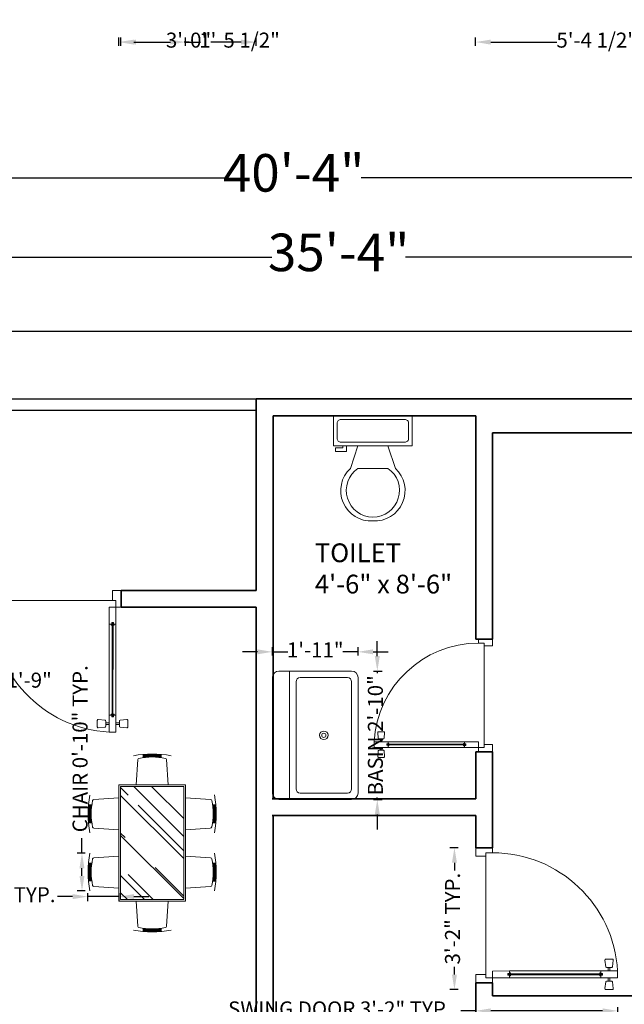
# Model space of a CAD drawing. Units: inches. Extents: x -638 to 186, y -762 to 59.
# Tile 21 of 31: x -287 to -125, y -203 to 59. Entities that reach past the tile are written whole.
import ezdxf

# ---------------------------------------------------------------- set-up
doc = ezdxf.new("R2010")
doc.units = ezdxf.units.IN
for name, color, linetype, lineweight in [('A-ANNO-DIMS', 2, 'Continuous', 18), ('A-AREA-IDEN', 1, 'Continuous', 18), ('A-DOOR', 3, 'Continuous', 18), ('A-FLOR-EDGE', 1, 'Continuous', 25), ('A-FLOR-FIXT', 9, 'Continuous', 18), ('A-FURN-PATT', 8, 'Continuous', 9), ('C-PROP', 7, 'Continuous', 25), ('furn', 8, 'Continuous', 13), ('wall', 7, 'Continuous', 35)]:
    doc.layers.add(name, color=color, linetype=linetype, lineweight=lineweight)
doc.styles.get("Standard").update_dxf_attribs({"font": 'arial.ttf'})
doc.dimstyles.new('ISO-25', dxfattribs={"dimtxt": 4, "dimasz": 4, "dimexe": 1.25, "dimexo": 0.625, "dimtad": 0, "dimlunit": 4, "dimtxsty": 'Standard', "dimcen": 2.5, "dimclrt": 256, "dimadec": 0, "dimazin": 0, "dimtfac": 1, "dimtmove": 0, "dimatfit": 3, "dimfxl": 1, "dimfxlon": 1, "dimarcsym": 0})

# ---------------------------------------------------------------- blocks, each defined once
blk = doc.blocks.new('*U4')
for p, q in [((9.5, -6), (9.5, -2)), ((-10, -8.5), (-8, -8.5)), ((-10, -9.5), (-10, -8.5)), ((-7, -9.5), (-10, -9.5)), ((-8, -8.5), (-8, -8)), ((-7, -8), (-7, -9.5)), ((-4, -8), (-6, -14)), ((4, -8), (6, -14)), ((4, -14), (-4, -14))]:
    blk.add_line(p, q)
blk.add_lwpolyline([(10.5, -8), (10.5, 0), (-10.5, 0), (-10.5, -8)], close=True)
for points in [[(-9.5, -2), (-9.5, -6)], [(8.5, -1), (-8.5, -1)], [(-8.5, -7), (8.5, -7)]]:
    blk.add_lwpolyline(points)
for centre, radius, start, end in [((-8.625, -1.875), 0.8839, 81.8699, 188.1301), ((8.625, -1.875), 0.8839, 351.8699, 98.1301), ((-8.625, -6.125), 0.8839, 171.869898, 278.1301), ((8.625, -6.125), 0.8839, 261.8699, 8.1301), ((-0.4772, -19.9188), 8.0953, 133.01722, 273.38), ((0.0374, -19.8731), 7.127, 124.50543, 269.7), ((-0.0373, -19.8731), 7.127, 270.3, 55.4946), ((0.4773, -19.9188), 8.0953, 266.62, 46.9828)]:
    blk.add_arc(centre, radius, start, end)
blk = doc.blocks.new('Sink-single - 30 in top')
blk.add_line((-15, -3.999996), (15, -3.999996))
for points in [[(-13.5, 0), (13.5, 0)], [(-15, -18.499996), (-15, -1.5)], [(15, -1.5), (15, -18.499996)], [(-13.5, -17.499996), (-13.5, -6.499996)], [(-12.5, -5.499996), (12.5, -5.499996)], [(13.5, -6.499996), (13.5, -17.499996)], [(13.5, -19.999996), (-13.5, -19.999996)], [(12.5, -18.499996), (-12.5, -18.499996)]]:
    blk.add_lwpolyline(points)
for radius in [1, 0.5]:
    blk.add_circle((0, -11.999996), radius)
for centre, radius, start, end in [((-13.5, -1.5), 1.5, 90, 180), ((13.5, -1.5), 1.5, 0, 90), ((-12.5, -6.499996), 1, 90, 180), ((12.5, -6.499996), 1, 0, 90), ((-12.5, -17.499996), 1, 180, 270), ((12.5, -17.499996), 1, 270, 0), ((-13.5, -18.499996), 1.5, 180, 270), ((13.5, -18.499996), 1.5, 270, 0)]:
    blk.add_arc(centre, radius, start, end)
blk = doc.blocks.new('*D9')
at = {"layer": 'A-ANNO-DIMS', "color": 0, "lineweight": -2, "transparency": 16777216}
for p, q in [((-413.53, -5.3), (-413.53, -3.05)), ((-403.53, -4.3), (-219.32, -4.3)), ((0.47, -4.3), (-183.73, -4.3)), ((10.47, -5.3), (10.47, -3.05))]:
    blk.add_line(p, q, dxfattribs=at)
at = {"layer": 'A-ANNO-DIMS', "color": 0, "lineweight": 30, "transparency": 16777216}
for points in [[(-403.53, -2.64), (-403.53, -5.97), (-413.53, -4.3)], [(0.47, -2.64), (0.47, -5.97), (10.47, -4.3)]]:
    blk.add_solid(points, dxfattribs=at)
at = {"layer": 'Defpoints', "color": 0, "lineweight": 30, "transparency": 16777216}
for p in [(10.47, -4.3), (-413.53, -42.03), (10.47, -42.03)]:
    blk.add_point(p, dxfattribs=at)
at = {"layer": 'A-ANNO-DIMS', "color": 0, "transparency": 16777216, "insert": (-201.53, -4.3), "char_height": 10, "attachment_point": 5}
blk.add_mtext('35\'-4"', dxfattribs=at)
blk = doc.blocks.new('*D11')
at = {"layer": 'A-ANNO-DIMS', "color": 0, "lineweight": -2, "transparency": 16777216}
for p, q in [((-455.53, 15.89), (-455.53, 18.14)), ((-445.53, 16.89), (-231.53, 16.89)), ((18.47, 16.89), (-195.52, 16.89)), ((28.47, 15.89), (28.47, 18.14))]:
    blk.add_line(p, q, dxfattribs=at)
at = {"layer": 'A-ANNO-DIMS', "color": 0, "lineweight": 30, "transparency": 16777216}
for points in [[(-445.53, 18.56), (-445.53, 15.23), (-455.53, 16.89)], [(18.47, 18.56), (18.47, 15.23), (28.47, 16.89)]]:
    blk.add_solid(points, dxfattribs=at)
at = {"layer": 'Defpoints', "color": 0, "lineweight": 30, "transparency": 16777216}
for p in [(28.47, 16.89), (-455.53, -42.03), (28.47, -42.03)]:
    blk.add_point(p, dxfattribs=at)
at = {"layer": 'A-ANNO-DIMS', "color": 0, "transparency": 16777216, "insert": (-213.53, 16.89), "char_height": 10, "attachment_point": 5}
blk.add_mtext('40\'-4"', dxfattribs=at)
blk = doc.blocks.new('DOOR-SWING-36IN')
for p, q in [((35.54, 35.1), (4.05, 35.09)), ((3.95, 4.05), (3.94, 29.24)), ((4.06, 4.05), (4.06, 29.24)), ((4.18, 4.05), (4.17, 29.24)), ((3.16, 4.5), (3.16, 28.79)), ((4.96, 4.5), (4.96, 28.79))]:
    blk.add_line(p, q)
for points in [[(3.16, 33.29), (3.15, 35.09), (4.05, 35.09), (4.05, 37.78), (1.8, 37.78), (1.81, 33.29), (3.16, 33.29)], [(36.44, 33.3), (36.44, 35.1), (35.54, 35.1), (35.54, 37.79), (37.79, 37.8), (37.79, 33.3), (36.44, 33.3)], [(4.28, 28.79), (4.96, 28.79), (4.95, 33.29), (3.16, 33.29), (3.16, 28.79), (3.83, 28.79), (3.83, 29.24), (4.28, 29.24), (4.28, 28.79)], [(4.29, 4.5), (4.96, 4.5), (4.96, 0), (3.17, 0), (3.16, 4.5), (3.84, 4.5), (3.84, 4.05), (4.29, 4.05), (4.29, 4.5)]]:
    blk.add_lwpolyline(points)
for points in [[(2.05, 3.17), (0.25, 3.35, 0.443716), (0, 3.12), (0, 1.37, 0.443716), (0.25, 1.15), (2.05, 1.33, 0.385314), (2.25, 1.55), (2.25, 2.94, 0.385314)], [(6.08, 3.17), (7.88, 3.35, -0.443716), (8.13, 3.13), (8.13, 1.37, -0.443716), (7.88, 1.15), (6.08, 1.33, -0.385314), (5.88, 1.55), (5.88, 2.95, -0.385314)]]:
    blk.add_lwpolyline(points, format="xyb", close=True)
for points in [[(3.16, 2.47), (2.25, 2.47), (2.25, 2.02), (3.17, 2.02)], [(4.96, 2.47), (5.88, 2.47), (5.88, 2.03), (4.96, 2.02)]]:
    blk.add_lwpolyline(points, close=True)
for centre, radius, start, end in [((3.06, 33.32), 33.38, 273.2653, 359.953), ((3.92, 28.83), 0.371, 186.4522, 273.3078), ((4.19, 28.83), 0.371, 266.7282, 353.5838), ((3.93, 4.46), 0.371, 86.7282, 173.5838), ((4.2, 4.46), 0.371, 6.4522, 93.3078)]:
    blk.add_arc(centre, radius, start, end)
blk = doc.blocks.new('DOOR-SWING-30IN')
for p, q in [((29.62, 29.25), (3.38, 29.24)), ((2.64, 3.75), (2.63, 23.99)), ((3.29, 3.37), (3.29, 24.37)), ((3.39, 3.37), (3.38, 24.37)), ((3.48, 3.37), (3.47, 24.37)), ((4.14, 3.75), (4.13, 23.99))]:
    blk.add_line(p, q)
for points in [[(2.63, 27.74), (2.63, 29.24), (3.38, 29.24), (3.38, 31.49), (1.5, 31.49), (1.51, 27.74), (2.63, 27.74)], [(30.37, 27.75), (30.37, 29.25), (29.62, 29.25), (29.62, 31.5), (31.5, 31.5), (31.5, 27.75), (30.37, 27.75)], [(3.57, 23.99), (4.13, 23.99), (4.13, 27.74), (2.63, 27.74), (2.63, 23.99), (3.19, 23.99), (3.19, 24.37), (3.57, 24.37), (3.57, 23.99)], [(3.57, 3.75), (4.14, 3.75), (4.14, 0), (2.64, 0), (2.64, 3.75), (3.2, 3.75), (3.2, 3.37), (3.57, 3.37), (3.57, 3.75)]]:
    blk.add_lwpolyline(points)
for points in [[(1.71, 2.64), (0.21, 2.79, 0.443716), (0, 2.6), (0, 1.14, 0.443716), (0.21, 0.96), (1.71, 1.11, 0.385314), (1.87, 1.29), (1.87, 2.45, 0.385314)], [(5.07, 2.64), (6.57, 2.79, -0.443716), (6.77, 2.61), (6.78, 1.15, -0.443716), (6.57, 0.96), (5.07, 1.11, -0.385314), (4.9, 1.3), (4.9, 2.46, -0.385314)]]:
    blk.add_lwpolyline(points, format="xyb", close=True)
for points in [[(2.64, 2.06), (1.87, 2.06), (1.87, 1.69), (2.64, 1.69)], [(4.14, 2.06), (4.9, 2.06), (4.9, 1.69), (4.14, 1.69)]]:
    blk.add_lwpolyline(points, close=True)
for centre, radius, start, end in [((2.55, 27.77), 27.82, 273.2653, 359.953), ((3.27, 24.03), 0.309, 186.4522, 273.3078), ((3.49, 24.03), 0.309, 266.7282, 353.5838), ((3.28, 3.71), 0.309, 86.7282, 173.5838), ((3.5, 3.71), 0.309, 6.4522, 93.3078)]:
    blk.add_arc(centre, radius, start, end)
blk = doc.blocks.new('CHAIR-DINING')
for p, q in [((2.65, 7.21), (2.65, 8.09)), ((2.87, 7.24), (2.87, 8.1)), ((3.09, 7.27), (3.09, 8.12)), ((3.31, 7.3), (3.31, 8.14)), ((3.53, 7.32), (3.53, 8.15)), ((3.75, 7.34), (3.75, 8.16)), ((3.98, 7.36), (3.98, 8.17)), ((4.2, 7.37), (4.2, 8.18)), ((4.42, 7.39), (4.42, 8.18)), ((4.64, 7.4), (4.64, 8.19)), ((4.86, 7.4), (4.86, 8.19)), ((5.03, 7.41), (5.03, 8.19)), ((5.19, 7.4), (5.19, 8.19)), ((5.41, 7.4), (5.41, 8.19)), ((5.64, 7.39), (5.64, 8.18)), ((5.86, 7.37), (5.86, 8.18)), ((6.08, 7.36), (6.08, 8.17)), ((6.3, 7.34), (6.3, 8.16)), ((6.52, 7.32), (6.52, 8.15)), ((6.74, 7.3), (6.74, 8.14)), ((6.96, 7.27), (6.96, 8.12)), ((7.19, 7.24), (7.19, 8.1)), ((7.41, 7.21), (7.41, 8.09)), ((0.77, 0), (1.22, 6.7)), ((9.29, 0), (8.83, 6.7))]:
    blk.add_line(p, q)
blk.add_lwpolyline([(10.05, 7.73, 0.091245), (0, 7.73, 0.091245)], format="xyb")
for centre, radius, start, end in [((1.55, 6.68), 0.332, 101.9645, 176.1255), ((5.35, -11.23), 18.64, 90.9862, 101.9645), ((4.71, -11.23), 18.64, 78.0355, 89.0138), ((8.5, 6.68), 0.332, 3.8745, 78.0355)]:
    blk.add_arc(centre, radius, start, end)
blk = doc.blocks.new('*D21')
at = {"layer": 'A-ANNO-DIMS', "color": 0, "lineweight": -2, "transparency": 16777216}
for p, q in [((-269.92, -163.03), (-269.92, -159.03)), ((-269.04, -163.03), (-271.17, -163.03)), ((-269.92, -169.09), (-269.92, -167.03)), ((-269.04, -173.09), (-271.17, -173.09))]:
    blk.add_line(p, q, dxfattribs=at)
at = {"layer": 'A-ANNO-DIMS', "color": 0, "lineweight": 30, "transparency": 16777216}
for points in [[(-270.59, -167.03), (-269.26, -167.03), (-269.92, -163.03)], [(-270.59, -169.09), (-269.26, -169.09), (-269.92, -173.09)]]:
    blk.add_solid(points, dxfattribs=at)
at = {"layer": 'Defpoints', "color": 0, "lineweight": 30, "transparency": 16777216}
for p in [(-269.92, -163.03), (-268.41, -163.03), (-268.41, -173.09)]:
    blk.add_point(p, dxfattribs=at)
at = {"layer": 'A-ANNO-DIMS', "transparency": 16777216, "insert": (-269.92, -135.22), "char_height": 4, "attachment_point": 5, "rotation": 90}
blk.add_mtext('CHAIR 0\'-10" TYP.', dxfattribs=at)
blk = doc.blocks.new('*D22')
at = {"layer": 'A-ANNO-DIMS', "color": 0, "lineweight": -2, "transparency": 16777216}
for p, q in [((-272.41, -174.6), (-276.41, -174.6)), ((-268.41, -173.71), (-268.41, -175.85)), ((-260.07, -174.6), (-268.41, -174.6)), ((-260.07, -173.71), (-260.07, -175.85)), ((-256.07, -174.6), (-252.07, -174.6))]:
    blk.add_line(p, q, dxfattribs=at)
at = {"layer": 'A-ANNO-DIMS', "color": 0, "lineweight": 30, "transparency": 16777216}
for points in [[(-272.41, -173.93), (-272.41, -175.26), (-268.41, -174.6)], [(-256.07, -173.93), (-256.07, -175.26), (-260.07, -174.6)]]:
    blk.add_solid(points, dxfattribs=at)
at = {"layer": 'Defpoints', "color": 0, "lineweight": 30, "transparency": 16777216}
for p in [(-268.41, -173.09), (-260.07, -173.09), (-268.41, -174.6)]:
    blk.add_point(p, dxfattribs=at)
at = {"layer": 'A-ANNO-DIMS', "transparency": 16777216, "insert": (-293.89, -174.6), "char_height": 4, "attachment_point": 5, "rotation": 360}
blk.add_mtext('0\'-8 1/2" TYP.', dxfattribs=at)
blk = doc.blocks.new('*D23')
at = {"layer": 'A-ANNO-DIMS', "color": 0, "lineweight": -2, "transparency": 16777216}
for p, q in [((-165.01, -204.03), (-165.01, -206.28)), ((-127.22, -204.03), (-127.22, -206.28)), ((-165.01, -205.03), (-169.01, -205.03)), ((-131.22, -205.03), (-161.01, -205.03))]:
    blk.add_line(p, q, dxfattribs=at)
at = {"layer": 'A-ANNO-DIMS', "color": 0, "lineweight": 30, "transparency": 16777216}
for points in [[(-161.01, -204.37), (-161.01, -205.7), (-165.01, -205.03)], [(-131.22, -204.37), (-131.22, -205.7), (-127.22, -205.03)]]:
    blk.add_solid(points, dxfattribs=at)
at = {"layer": 'Defpoints', "color": 0, "lineweight": 30, "transparency": 16777216}
for p in [(-165.01, -199.36), (-127.22, -199.36), (-165.01, -205.03)]:
    blk.add_point(p, dxfattribs=at)
at = {"layer": 'A-ANNO-DIMS', "transparency": 16777216, "insert": (-201.22, -205.03), "char_height": 4, "attachment_point": 5}
blk.add_mtext('SWING DOOR 3\'-2" TYP.', dxfattribs=at)
blk = doc.blocks.new('*D24')
at = {"layer": 'A-ANNO-DIMS', "color": 0, "lineweight": -2, "transparency": 16777216}
for p, q in [((-169.68, -161.57), (-171.93, -161.57)), ((-170.68, -165.57), (-170.68, -167.65)), ((-170.68, -195.36), (-170.68, -193.28)), ((-169.68, -199.36), (-171.93, -199.36))]:
    blk.add_line(p, q, dxfattribs=at)
at = {"layer": 'A-ANNO-DIMS', "color": 0, "lineweight": 30, "transparency": 16777216}
for points in [[(-171.35, -165.57), (-170.02, -165.57), (-170.68, -161.57)], [(-171.35, -195.36), (-170.02, -195.36), (-170.68, -199.36)]]:
    blk.add_solid(points, dxfattribs=at)
at = {"layer": 'Defpoints', "color": 0, "lineweight": 30, "transparency": 16777216}
for p in [(-170.68, -161.57), (-165.01, -161.57), (-165.01, -199.36)]:
    blk.add_point(p, dxfattribs=at)
at = {"layer": 'A-ANNO-DIMS', "transparency": 16777216, "insert": (-170.68, -180.47), "char_height": 4, "attachment_point": 5, "rotation": 90}
blk.add_mtext('3\'-2" TYP.', dxfattribs=at)
blk = doc.blocks.new('*D31')
at = {"layer": 'A-ANNO-DIMS', "color": 0, "lineweight": -2, "transparency": 16777216}
for p, q in [((-191.23, -110.53), (-191.23, -106.53)), ((-192.23, -114.53), (-189.98, -114.53)), ((-191.23, -114.53), (-191.23, -115.06)), ((-192.23, -148.73), (-189.98, -148.73)), ((-191.23, -148.73), (-191.23, -148.2)), ((-191.23, -152.73), (-191.23, -156.73))]:
    blk.add_line(p, q, dxfattribs=at)
at = {"layer": 'A-ANNO-DIMS', "color": 0, "lineweight": 30, "transparency": 16777216}
for points in [[(-191.9, -110.53), (-190.57, -110.53), (-191.23, -114.53)], [(-191.9, -152.73), (-190.57, -152.73), (-191.23, -148.73)]]:
    blk.add_solid(points, dxfattribs=at)
at = {"layer": 'Defpoints', "color": 0, "lineweight": 30, "transparency": 16777216}
for p in [(-196.36, -114.53), (-191.23, -114.53), (-196.36, -148.73)]:
    blk.add_point(p, dxfattribs=at)
at = {"layer": 'A-ANNO-DIMS', "transparency": 16777216, "insert": (-191.23, -131.63), "char_height": 4, "attachment_point": 5, "rotation": 90}
blk.add_mtext('BASIN 2\'-10"', dxfattribs=at)
blk = doc.blocks.new('*D32')
at = {"layer": 'A-ANNO-DIMS', "color": 0, "lineweight": -2, "transparency": 16777216}
for p, q in [((-223.17, -109.4), (-227.17, -109.4)), ((-219.17, -110.4), (-219.17, -108.15)), ((-219.17, -109.4), (-215.07, -109.4)), ((-196.36, -109.4), (-200.46, -109.4)), ((-196.36, -110.4), (-196.36, -108.15)), ((-192.36, -109.4), (-188.36, -109.4))]:
    blk.add_line(p, q, dxfattribs=at)
at = {"layer": 'A-ANNO-DIMS', "color": 0, "lineweight": 30, "transparency": 16777216}
for points in [[(-223.17, -108.73), (-223.17, -110.06), (-219.17, -109.4)], [(-192.36, -108.73), (-192.36, -110.06), (-196.36, -109.4)]]:
    blk.add_solid(points, dxfattribs=at)
at = {"layer": 'Defpoints', "color": 0, "lineweight": 30, "transparency": 16777216}
for p in [(-219.17, -109.4), (-219.17, -114.53), (-196.36, -114.53)]:
    blk.add_point(p, dxfattribs=at)
at = {"layer": 'A-ANNO-DIMS', "transparency": 16777216, "insert": (-207.77, -109.4), "char_height": 4, "attachment_point": 5}
blk.add_mtext('1\'-11"', dxfattribs=at)
blk = doc.blocks.new('*D48')
at = {"layer": 'A-ANNO-DIMS', "color": 0, "lineweight": -2, "transparency": 16777216}
for p, q in [((-260.07, 52.02), (-260.07, 54.27)), ((-256.07, 53.02), (-246.35, 53.02)), ((-242.35, 52.02), (-242.35, 54.27)), ((-242.35, 53.02), (-238.35, 53.02))]:
    blk.add_line(p, q, dxfattribs=at)
at = {"layer": 'A-ANNO-DIMS', "color": 0, "lineweight": 30, "transparency": 16777216}
for points in [[(-256.07, 53.68), (-256.07, 52.35), (-260.07, 53.02)], [(-246.35, 53.68), (-246.35, 52.35), (-242.35, 53.02)]]:
    blk.add_solid(points, dxfattribs=at)
at = {"layer": 'Defpoints', "color": 0, "lineweight": 30, "transparency": 16777216}
for p in [(-242.35, 53.02), (-260.07, -144.8), (-242.35, -144.8)]:
    blk.add_point(p, dxfattribs=at)
at = {"layer": 'A-ANNO-DIMS', "transparency": 16777216, "insert": (-227.94, 53.02), "char_height": 4, "attachment_point": 5}
blk.add_mtext('1\'-5 1/2"', dxfattribs=at)
blk = doc.blocks.new('*D49')
at = {"layer": 'A-ANNO-DIMS', "color": 0, "lineweight": -2, "transparency": 16777216}
for p, q in [((182.66, -144.8), (184.91, -144.8)), ((183.66, -148.8), (183.66, -154.33)), ((183.66, -171.81), (183.66, -166.28)), ((182.66, -175.81), (184.91, -175.81))]:
    blk.add_line(p, q, dxfattribs=at)
at = {"layer": 'A-ANNO-DIMS', "color": 0, "lineweight": 30, "transparency": 16777216}
for points in [[(183, -148.8), (184.33, -148.8), (183.66, -144.8)], [(183, -171.81), (184.33, -171.81), (183.66, -175.81)]]:
    blk.add_solid(points, dxfattribs=at)
at = {"layer": 'Defpoints', "color": 0, "lineweight": 30, "transparency": 16777216}
for p in [(-242.35, -144.8), (-242.35, -175.81), (183.66, -175.81)]:
    blk.add_point(p, dxfattribs=at)
at = {"layer": 'A-ANNO-DIMS', "transparency": 16777216, "insert": (183.66, -160.31), "char_height": 4, "attachment_point": 5, "rotation": 90}
blk.add_mtext('2\'-7"', dxfattribs=at)
blk = doc.blocks.new('*D55')
at = {"layer": 'A-ANNO-DIMS', "color": 0, "lineweight": -2, "transparency": 16777216}
for p, q in [((-259.53, 52.02), (-259.53, 54.27)), ((-255.53, 53.02), (-247.47, 53.02)), ((-227.53, 53.02), (-235.59, 53.02)), ((-223.53, 52.02), (-223.53, 54.27))]:
    blk.add_line(p, q, dxfattribs=at)
at = {"layer": 'A-ANNO-DIMS', "color": 0, "lineweight": 30, "transparency": 16777216}
for points in [[(-255.53, 53.68), (-255.53, 52.35), (-259.53, 53.02)], [(-227.53, 53.68), (-227.53, 52.35), (-223.53, 53.02)]]:
    blk.add_solid(points, dxfattribs=at)
at = {"layer": 'Defpoints', "color": 0, "lineweight": 30, "transparency": 16777216}
for p in [(-259.53, 53.02), (-259.53, -97.53), (-223.53, -97.53)]:
    blk.add_point(p, dxfattribs=at)
at = {"layer": 'A-ANNO-DIMS', "transparency": 16777216, "insert": (-241.53, 53.02), "char_height": 4, "attachment_point": 5}
blk.add_mtext('3\'-0"', dxfattribs=at)
blk = doc.blocks.new('*D56')
at = {"layer": 'A-ANNO-DIMS', "color": 0, "lineweight": -2, "transparency": 16777216}
for p, q in [((-165.03, 52.02), (-165.03, 54.27)), ((-161.03, 53.02), (-143.38, 53.02)), ((-104.53, 53.02), (-122.17, 53.02)), ((-100.53, 52.02), (-100.53, 54.27))]:
    blk.add_line(p, q, dxfattribs=at)
at = {"layer": 'A-ANNO-DIMS', "color": 0, "lineweight": 30, "transparency": 16777216}
for points in [[(-161.03, 53.68), (-161.03, 52.35), (-165.03, 53.02)], [(-104.53, 53.68), (-104.53, 52.35), (-100.53, 53.02)]]:
    blk.add_solid(points, dxfattribs=at)
at = {"layer": 'Defpoints', "color": 0, "lineweight": 30, "transparency": 16777216}
for p in [(-100.53, 53.02), (-165.03, -408.03), (-100.53, -408.03)]:
    blk.add_point(p, dxfattribs=at)
at = {"layer": 'A-ANNO-DIMS', "transparency": 16777216, "insert": (-132.78, 53.02), "char_height": 4, "attachment_point": 5}
blk.add_mtext('5\'-4 1/2"', dxfattribs=at)
blk = doc.blocks.new('*D58')
at = {"layer": 'A-ANNO-DIMS', "color": 0, "lineweight": -2, "transparency": 16777216}
for p, q in [((-330.45, -117.46), (-309.6, -117.46)), ((-301.6, -117.46), (-305.6, -117.46))]:
    blk.add_line(p, q, dxfattribs=at)
at = {"layer": 'A-ANNO-DIMS', "color": 0, "lineweight": 30, "transparency": 16777216}
blk.add_solid([(-305.6, -116.8), (-305.6, -118.13), (-309.6, -117.46)], dxfattribs=at)
at = {"layer": 'Defpoints', "color": 0, "lineweight": 30, "transparency": 16777216}
for p in [(-330.45, -117.46), (-309.6, -117.46)]:
    blk.add_point(p, dxfattribs=at)
at = {"layer": 'A-ANNO-DIMS', "transparency": 16777216, "insert": (-289.42, -117.46), "char_height": 4, "attachment_point": 5, "rotation": 0.0013}
blk.add_mtext('2X R1\'-9"', dxfattribs=at)

msp = doc.modelspace()

# ---------------------------------------------------------------- hatches: boundary and pattern name
at = {"layer": 'A-FURN-PATT'}
h = msp.add_hatch(dxfattribs=at)
h.set_pattern_fill('AR-RROOF', color=256, scale=0.442997, angle=135, style=0)
h.set_pattern_definition([(135, (126.657, -989.558), (-25.46067, 9.54775), [168.782, -22.5043, 56.2607, -11.2521]), (135, (112.096, -982.954), (-2.62563, -18.53855), [33.7564, -3.7132, 67.5128, -8.4391]), (135, (115.9155, -992.343), (-46.704425, 36.04277), [90.0171, -15.753, 45.00854, -11.25213])])
h.paths.add_polyline_path([(-259.629, -175.37), (-242.795, -175.37), (-242.795, -145.246), (-259.629, -145.246)])

# ---------------------------------------------------------------- linework, layer by layer
at = {"layer": 'A-FLOR-EDGE'}
for p, q in [((-413.526, -42.033), (-223.526, -42.033)), ((-413.526, -45.033), (-223.526, -45.033))]:
    msp.add_line(p, q, dxfattribs=at)
at = {"layer": 'C-PROP'}
msp.add_line((10.474, -24.033), (-468.465, -24.033), dxfattribs=at)
at = {"layer": 'furn'}
for p, q in [((-242.352, -148.296), (-235.65, -148.75)), ((-235.14, -150.175), (-234.266, -150.175)), ((-235.109, -150.397), (-234.248, -150.397)), ((-235.08, -150.618), (-234.231, -150.618)), ((-235.055, -150.84), (-234.217, -150.84)), ((-235.032, -151.061), (-234.204, -151.061)), ((-235.011, -151.283), (-234.193, -151.283)), ((-234.994, -151.504), (-234.184, -151.504)), ((-234.979, -151.726), (-234.176, -151.726)), ((-234.966, -151.947), (-234.17, -151.947)), ((-235.109, -154.715), (-234.248, -154.715)), ((-235.08, -154.493), (-234.231, -154.493)), ((-235.055, -154.272), (-234.217, -154.272)), ((-235.032, -154.05), (-234.204, -154.05)), ((-235.011, -153.829), (-234.193, -153.829)), ((-234.994, -153.607), (-234.184, -153.607)), ((-234.979, -153.386), (-234.176, -153.386)), ((-234.966, -153.164), (-234.17, -153.164)), ((-234.956, -152.169), (-234.167, -152.169)), ((-234.956, -152.943), (-234.167, -152.943)), ((-234.949, -152.39), (-234.164, -152.39)), ((-234.949, -152.721), (-234.164, -152.721)), ((-234.946, -152.556), (-234.164, -152.556)), ((-242.352, -156.815), (-235.734, -156.367)), ((-235.14, -154.936), (-234.266, -154.936))]:
    msp.add_line(p, q, dxfattribs=at)
for points in [[(-242.352, -175.813), (-242.352, -144.803), (-260.072, -144.803), (-260.072, -175.813)], [(-242.795, -175.37), (-242.795, -145.246), (-259.629, -145.246), (-259.629, -175.37)]]:
    msp.add_lwpolyline(points, close=True, dxfattribs=at)
msp.add_lwpolyline([(-234.622, -147.529, -0.0912453), (-234.622, -157.582, -0.0912453)], format="xyb", dxfattribs=at)
for centre, radius, start, end in [((-235.673, -149.082), 0.332, 11.96453, 86.12552), ((-253.579, -152.876), 18.636, 0.98618, 11.96453), ((-253.579, -152.235), 18.636, 348.29889, 359.01382), ((-235.764, -155.925), 0.443, 273.87448, 348.29889)]:
    msp.add_arc(centre, radius, start, end, dxfattribs=at)
at = {"layer": 'wall'}
for p, q in [((-223.526, -42.033), (10.474, -42.033)), ((-223.526, -93.033), (-223.526, -42.033)), ((-219.026, -46.533), (-165.026, -46.533)), ((-165.026, -46.533), (-219.026, -46.533)), ((-219.026, -46.533), (-219.026, -148.533)), ((-165.026, -46.533), (-165.026, -105.991)), ((-160.526, -51.033), (-160.526, -105.991)), ((-160.526, -51.033), (1.474, -51.033)), ((-160.526, -51.033), (1.474, -51.033)), ((-259.526, -97.533), (-259.526, -93.033)), ((-259.526, -93.033), (-223.526, -93.033)), ((-223.526, -97.533), (-259.526, -97.533)), ((-259.526, -97.533), (-223.526, -97.533)), ((-223.526, -210.033), (-223.526, -97.533)), ((-165.026, -105.991), (-160.526, -105.991)), ((-165.026, -135.991), (-160.526, -135.991)), ((-165.026, -135.991), (-165.026, -148.525)), ((-160.526, -135.991), (-160.526, -161.592)), ((-219.255, -148.525), (-165.026, -148.525)), ((-219.026, -148.533), (-165.026, -148.533)), ((-219.255, -153.025), (-165.026, -153.025)), ((-219.026, -214.533), (-219.026, -153.025)), ((-219.026, -153.033), (-219.026, -153.025)), ((-165.026, -153.025), (-165.026, -161.592)), ((-165.026, -153.025), (-165.026, -153.033)), ((-160.526, -161.592), (-165.026, -161.592)), ((-160.526, -197.592), (-165.026, -197.592)), ((-165.026, -197.592), (-165.026, -354.033)), ((-160.526, -197.592), (-160.526, -201.033)), ((-160.526, -201.033), (1.474, -201.033))]:
    msp.add_line(p, q, dxfattribs=at)

# ---------------------------------------------------------------- block references
at = {"layer": 'A-DOOR', "extrusion": (0, 0, -1), "zscale": -1}
for name, p, xscale, yscale, rotation in [('DOOR-SWING-36IN', (257.711, -130.779), 0.9990020536126122, 0.9990020536126122, 359.9819968737387), ('DOOR-SWING-30IN', (192.074, -137.507), 1.001806283710001, 1.001806283710001, 89.98199687371395)]:
    msp.add_blockref(name, p, dxfattribs=dict(at, xscale=xscale, yscale=yscale, rotation=rotation))
at = {"layer": 'A-DOOR', "rotation": 89.99999999999973}
msp.add_blockref('DOOR-SWING-36IN', (-127.219, -199.363), dxfattribs=at)
at = {"layer": 'A-FLOR-FIXT'}
msp.add_blockref('*U4', (-192.413, -46.533), dxfattribs=at)
at = {"layer": 'A-FLOR-FIXT', "xscale": 1.14017526138166, "yscale": 1.14017526138166, "zscale": 1.14017526138166, "rotation": 90}
msp.add_blockref('Sink-single - 30 in top', (-219.167, -131.632), dxfattribs=at)
at = {"layer": 'furn'}
msp.add_blockref('CHAIR-DINING', (-256.239, -144.803), dxfattribs=at)
for p, rotation in [((-260.072, -157.582), 90.00000000180098), ((-260.072, -173.087), 89.99999999775004), ((-242.352, -163.034), 269.9999999963203), ((-246.186, -175.813), 180)]:
    msp.add_blockref('CHAIR-DINING', p, dxfattribs=dict(at, rotation=rotation))

# ---------------------------------------------------------------- texts
at = {"layer": 'A-AREA-IDEN', "insert": (-207.871, -80.517), "char_height": 5, "attachment_point": 1}
msp.add_mtext_dynamic_manual_height_columns('\\A1;{TOILET\\P4\'-6\\H1x;" x 8\'-6"}', width=99.04816, gutter_width=12.5, heights=[0], dxfattribs=at)

# ---------------------------------------------------------------- dimensions: what is measured, and where the dimension line sits
at = {"layer": 'A-ANNO-DIMS'}
for base, p1, p2, override, picture, middle in [((-242.352, 53.017), (-260.072, -144.803), (-242.352, -144.803), {"dimdec": 1, "dimlfac": 1, "dimrnd": 0, "dimzin": 1, "dimdsep": 46, "dimlunit": 4, "dimfrac": 2}, '*D48', (-227.939, 53.017)), ((-100.526, 53.017), (-165.026, -408.033), (-100.526, -408.033), {"dimdec": 1, "dimlfac": 1, "dimrnd": 0, "dimzin": 1, "dimdsep": 46, "dimlunit": 4, "dimfrac": 2}, '*D56', (-132.776, 53.017)), ((-259.526, 53.017), (-223.526, -97.533), (-259.526, -97.527), {"dimdec": 1, "dimlfac": 1, "dimrnd": 0, "dimzin": 1, "dimdsep": 46, "dimlunit": 4, "dimfrac": 2}, '*D55', (-241.526, 53.017)), ((28.474, 16.893), (-455.526, -42.033), (28.474, -42.033), {"dimtxt": 10, "dimasz": 10, "dimclrd": 0, "dimclre": 0, "dimclrt": 0}, '*D11', (-213.526, 16.893)), ((10.474, -4.303), (-413.526, -42.033), (10.474, -42.033), {"dimtxt": 10, "dimasz": 10, "dimclrd": 0, "dimclre": 0, "dimclrt": 0}, '*D9', (-201.526, -4.303))]:
    dim = msp.add_linear_dim(base=base, p1=p1, p2=p2, dimstyle='ISO-25', override=override, dxfattribs=at)
    dim.commit()
    dim.dimension.update_dxf_attribs({"geometry": picture, "text_midpoint": middle})
for base, p1, p2, angle, picture, middle in [((-219.167, -109.398), (-196.364, -114.529), (-219.167, -114.529), 180, '*D32', (-207.765, -109.398)), ((183.663, -175.813), (-242.352, -144.803), (-242.352, -175.813), 90, '*D49', (183.663, -160.308))]:
    dim = msp.add_linear_dim(base=base, p1=p1, p2=p2, angle=angle, dimstyle='ISO-25', override={"dimdec": 1, "dimlfac": 1, "dimrnd": 0, "dimzin": 1, "dimdsep": 46, "dimlunit": 4, "dimfrac": 2}, dxfattribs=at)
    dim.commit()
    dim.dimension.update_dxf_attribs({"geometry": picture, "text_midpoint": middle})
for base, p1, p2, angle, text, picture, middle in [((-191.233, -114.529), (-196.364, -148.734), (-196.364, -114.529), 90, 'BASIN <>', '*D31', (-191.233, -131.632)), ((-269.922, -163.034), (-268.414, -173.087), (-268.414, -163.034), 90, 'CHAIR <> TYP.', '*D21', (-269.922, -135.218)), ((-170.684, -161.572), (-165.015, -199.363), (-165.015, -161.572), 90, '<> TYP.', '*D24', (-170.684, -180.467)), ((-268.414, -174.595), (-260.072, -173.087), (-268.414, -173.087), 180, '<> TYP.', '*D22', (-293.89, -174.595)), ((-165.015, -205.032), (-127.219, -199.363), (-165.015, -199.363), 180, 'SWING DOOR <> TYP.', '*D23', (-201.224, -205.032))]:
    dim = msp.add_linear_dim(base=base, p1=p1, p2=p2, angle=angle, text=text, dimstyle='ISO-25', override={"dimdec": 1, "dimlfac": 1, "dimrnd": 0, "dimzin": 1, "dimdsep": 46, "dimlunit": 4, "dimfrac": 2}, dxfattribs=at)
    dim.commit()
    dim.dimension.update_dxf_attribs({"geometry": picture, "text_midpoint": middle})
dim = msp.add_radius_dim(center=(-330.447, -117.462), mpoint=(-309.605, -117.462), text='2X <>', dimstyle='ISO-25', override={"dimdec": 1, "dimlfac": 1, "dimrnd": 0, "dimzin": 1, "dimdsep": 46, "dimlunit": 4, "dimfrac": 2}, dxfattribs=at)
dim.commit()
dim.dimension.update_dxf_attribs({"geometry": '*D58', "text_midpoint": (-289.417, -117.462)})

doc.saveas('drawing.dxf')
